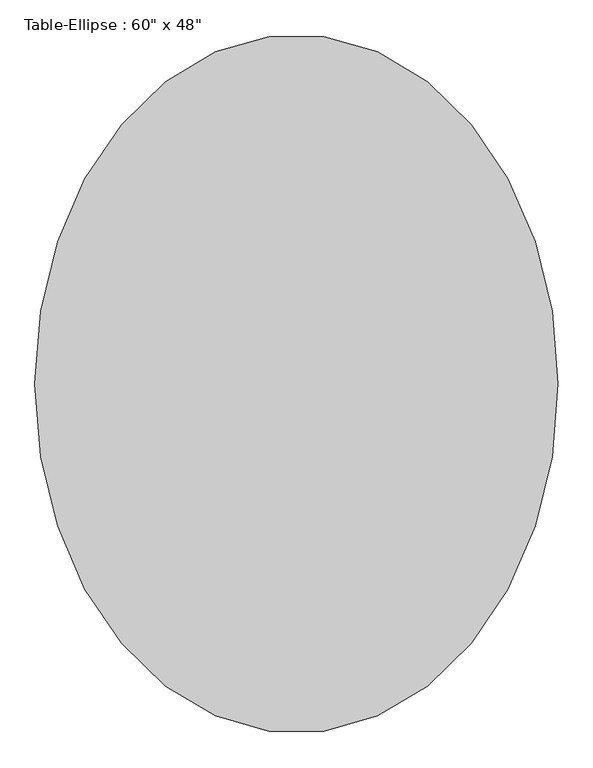
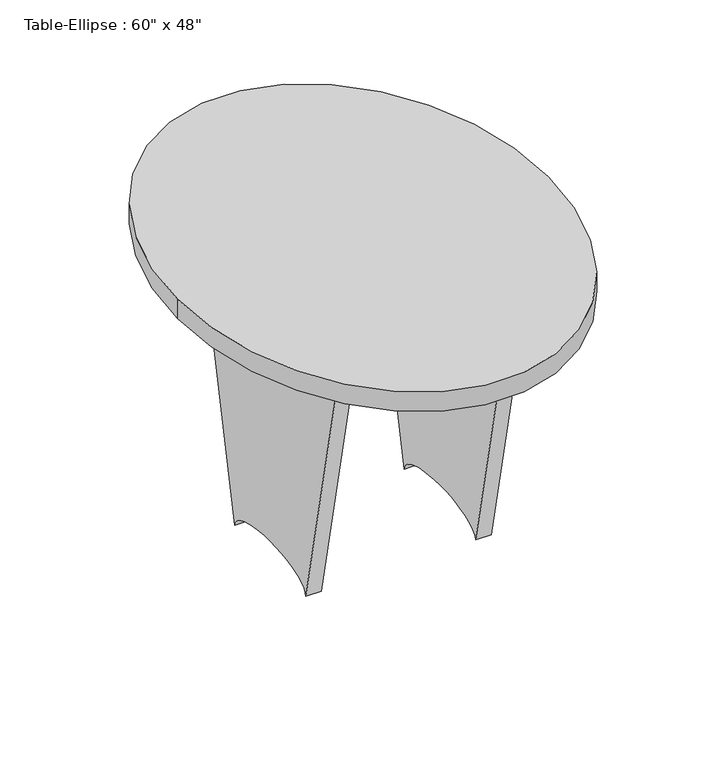
"""IFC4 building model written with IfcOpenShell, lengths in millimetres: furniture geometry."""

from ifc_helpers import new_model, si_unit, point, frame, origin, place, context, project, spatial, ellipse_curve, trimmed, source, transform, mapped, element, save
from ifc_brep_helpers import plane_surface, extruded_surface, advanced_brep


def furniture_b1c544a7(model_context):
    return source(origin(), model_context, "Body", "AdvancedBrep", [
        advanced_brep(
        [(-190.5, 19.05, 711.2), (190.5, 19.05, 711.2), (190.5, 19.05, 474.1333333), (-190.5, 19.05, 474.1333333), (-190.5, -19.05, 711.2), (-190.5, -19.05, 474.1333333), (190.5, -19.05, 474.1333333), (190.5, -19.05, 711.2)],
        [
            (0, 1),
            (1, 2),
            (2, 3, ellipse_curve(frame((0.0, 19.05, 474.1333333), z_axis=(0.0, -1.0, 0.0), x_axis=(1.0, 0.0, 0.0)), 190.5, 101.6)),
            (3, 0),
            (4, 5),
            (5, 6, ellipse_curve(frame((0.0, -19.05, 474.1333333), z_axis=(0.0, 1.0, 0.0), x_axis=(1.0, 0.0, 0.0)), 190.5, 101.6)),
            (6, 7),
            (7, 4),
            (0, 4),
            (7, 1),
            (6, 2),
            (5, 3),
        ],
        [
            plane_surface(frame((-190.5, 19.05, 711.2), z_axis=(0.0, 1.0, 0.0), x_axis=(1.0, 0.0, 0.0))),
            plane_surface(frame((-190.5, -19.05, 711.2), z_axis=(0.0, -1.0, 0.0), x_axis=(-1.0, 0.0, 0.0))),
            plane_surface(frame((-190.5, 19.05, 711.2), z_axis=(0.0, 0.0, 1.0), x_axis=(0.0, -1.0, 0.0))),
            plane_surface(frame((190.5, 19.05, 711.2), z_axis=(1.0, 0.0, 0.0), x_axis=(0.0, -1.0, 0.0))),
            extruded_surface(trimmed(ellipse_curve(frame((0.0, -57.15, 474.1333333), z_axis=(0.0, -1.0, 0.0), x_axis=(1.0, 0.0, 0.0)), 190.5, 101.6), [point((190.5, -57.15, 474.1333333))], [point((-190.5, -57.15, 474.1333333))], True, "CARTESIAN"), (0.0, 38.099999999999994, 0.0), 38.099999999999994),
            plane_surface(frame((-190.5, 19.05, 474.1333333), z_axis=(-1.0, 0.0, 0.0), x_axis=(0.0, -1.0, 0.0))),
        ],
        [
            (0, [[1, 2, 3, 4]]),
            (1, [[5, 6, 7, 8]]),
            (2, [[-1, 9, -8, 10]]),
            (3, [[-2, -10, -7, 11]]),
            (4, [[-3, -11, -6, 12]]),
            (5, [[-4, -12, -5, -9]]),
        ],
    ),
        advanced_brep(
        [(228.6, 304.8, 711.2), (228.6, -304.8, 711.2), (228.6, -152.4, 0.0), (228.6, 152.4, 0.0), (190.5, 304.8, 711.2), (190.5, 152.4, 0.0), (190.5, -152.4, 0.0), (190.5, -304.8, 711.2)],
        [
            (0, 1),
            (1, 2),
            (2, 3, ellipse_curve(frame((228.6, 0.0, 0.0), z_axis=(-1.0, 0.0, 0.0), x_axis=(0.0, 1.0, 0.0)), 152.4, 50.8)),
            (3, 0),
            (4, 5),
            (5, 6, ellipse_curve(frame((190.5, 0.0, 0.0), z_axis=(1.0, 0.0, 0.0), x_axis=(0.0, 1.0, 0.0)), 152.4, 50.8)),
            (6, 7),
            (7, 4),
            (0, 4),
            (7, 1),
            (6, 2),
            (5, 3),
        ],
        [
            plane_surface(frame((228.6, -304.8, 711.2), z_axis=(1.0, 0.0, 0.0), x_axis=(0.0, -1.0, 0.0))),
            plane_surface(frame((190.5, -304.8, 711.2), z_axis=(-1.0, 0.0, 0.0), x_axis=(0.0, 1.0, 0.0))),
            plane_surface(frame((228.6, 304.8, 711.2), z_axis=(0.0, 0.0, 1.0), x_axis=(-1.0, 0.0, 0.0))),
            plane_surface(frame((228.6, -304.8, 711.2), z_axis=(0.0, -0.9778024140774091, -0.2095290887308754), x_axis=(-1.0, 0.0, 0.0))),
            extruded_surface(trimmed(ellipse_curve(frame((152.4, 0.0, 0.0), z_axis=(-1.0, 0.0, 0.0), x_axis=(0.0, 1.0, 0.0)), 152.4, 50.8), [point((152.4, -152.4, 0.0))], [point((152.4, 152.4, 0.0))], True, "CARTESIAN"), (38.099999999999994, 0.0, 0.0), 38.099999999999994),
            plane_surface(frame((228.6, 152.4, 0.0), z_axis=(0.0, 0.977802414077412, -0.2095290887308621), x_axis=(-1.0, 0.0, 0.0))),
        ],
        [
            (0, [[1, 2, 3, 4]]),
            (1, [[5, 6, 7, 8]]),
            (2, [[-1, 9, -8, 10]]),
            (3, [[-2, -10, -7, 11]]),
            (4, [[-3, -11, -6, 12]]),
            (5, [[-4, -12, -5, -9]]),
        ],
    ),
        advanced_brep(
        [(-190.5, 304.8, 711.2), (-190.5, -304.8, 711.2), (-190.5, -152.4, 0.0), (-190.5, 152.4, 0.0), (-228.6, 304.8, 711.2), (-228.6, 152.4, 0.0), (-228.6, -152.4, 0.0), (-228.6, -304.8, 711.2)],
        [
            (0, 1),
            (1, 2),
            (2, 3, ellipse_curve(frame((-190.5, 0.0, 0.0), z_axis=(-1.0, 0.0, 0.0), x_axis=(0.0, 1.0, 0.0)), 152.4, 50.8)),
            (3, 0),
            (4, 5),
            (5, 6, ellipse_curve(frame((-228.6, 0.0, 0.0), z_axis=(1.0, 0.0, 0.0), x_axis=(0.0, 1.0, 0.0)), 152.4, 50.8)),
            (6, 7),
            (7, 4),
            (0, 4),
            (7, 1),
            (6, 2),
            (5, 3),
        ],
        [
            plane_surface(frame((-190.5, -304.8, 711.2), z_axis=(1.0, 0.0, 0.0), x_axis=(0.0, -1.0, 0.0))),
            plane_surface(frame((-228.6, -304.8, 711.2), z_axis=(-1.0, 0.0, 0.0), x_axis=(0.0, 1.0, 0.0))),
            plane_surface(frame((-190.5, 304.8, 711.2), z_axis=(0.0, 0.0, 1.0), x_axis=(-1.0, 0.0, 0.0))),
            plane_surface(frame((-190.5, -304.8, 711.2), z_axis=(0.0, -0.9778024140774088, -0.2095290887308767), x_axis=(-1.0, 0.0, 0.0))),
            extruded_surface(trimmed(ellipse_curve(frame((-266.7, 0.0, 0.0), z_axis=(-1.0, 0.0, 0.0), x_axis=(0.0, 1.0, 0.0)), 152.4, 50.8), [point((-266.7, -152.4, 0.0))], [point((-266.7, 152.4, 0.0))], True, "CARTESIAN"), (38.099999999999994, 0.0, 0.0), 38.099999999999994),
            plane_surface(frame((-190.5, 152.4, 0.0), z_axis=(0.0, 0.9778024140774109, -0.2095290887308677), x_axis=(-1.0, 0.0, 0.0))),
        ],
        [
            (0, [[1, 2, 3, 4]]),
            (1, [[5, 6, 7, 8]]),
            (2, [[-1, 9, -8, 10]]),
            (3, [[-2, -10, -7, 11]]),
            (4, [[-3, -11, -6, 12]]),
            (5, [[-4, -12, -5, -9]]),
        ],
    ),
        advanced_brep(
        [(-457.2, 0.0, 762.0), (457.2, 0.0, 762.0), (-457.2, 0.0, 711.2), (457.2, 0.0, 711.2)],
        [
            (0, 1, ellipse_curve(frame((0.0, 0.0, 762.0), z_axis=(0.0, 0.0, 1.0), x_axis=(0.0, 1.0, 0.0)), 609.6, 457.2)),
            (1, 0, ellipse_curve(frame((0.0, 0.0, 762.0), z_axis=(0.0, 0.0, 1.0), x_axis=(0.0, 1.0, 0.0)), 609.6, 457.2)),
            (2, 3, ellipse_curve(frame((0.0, 0.0, 711.2), z_axis=(0.0, 0.0, -1.0), x_axis=(1.0, 0.0, 0.0)), 457.2, 609.6)),
            (3, 2, ellipse_curve(frame((0.0, 0.0, 711.2), z_axis=(0.0, 0.0, -1.0), x_axis=(1.0, 0.0, 0.0)), 457.2, 609.6)),
            (0, 2),
            (3, 1),
        ],
        [
            plane_surface(frame((457.2, 0.0, 762.0), z_axis=(0.0, 0.0, 1.0), x_axis=(0.0, 1.0, 0.0))),
            plane_surface(frame((457.2, 0.0, 711.2), z_axis=(0.0, 0.0, -1.0), x_axis=(0.0, -1.0, 0.0))),
            extruded_surface(trimmed(ellipse_curve(frame((0.0, 0.0, 660.4), z_axis=(0.0, 0.0, 1.0), x_axis=(1.0, 0.0, 0.0)), 457.2, 609.6), [point((-457.2, 0.0, 660.4))], [point((457.2, 0.0, 660.4))], True, "CARTESIAN"), (0.0, 0.0, 50.80000000000007), 50.80000000000007),
            extruded_surface(trimmed(ellipse_curve(frame((0.0, 0.0, 660.4), z_axis=(0.0, 0.0, 1.0), x_axis=(1.0, 0.0, 0.0)), 457.2, 609.6), [point((457.2, 0.0, 660.4))], [point((-457.2, 0.0, 660.4))], True, "CARTESIAN"), (0.0, 0.0, 50.80000000000007), 50.80000000000007),
        ],
        [
            (0, [[1, 2]]),
            (1, [[3, 4]]),
            (2, [[-1, 5, -4, 6]]),
            (3, [[-2, -6, -3, -5]]),
        ],
    ),
    ])


if __name__ == "__main__":
    model = new_model("IFC4")
    model_context = context("Model", 3, world=origin())
    ifc_project = project(units=[si_unit("LENGTHUNIT", "METRE", prefix="MILLI")], contexts=[model_context])
    site = spatial("IfcSite", under=ifc_project)
    building = spatial("IfcBuilding", under=site)
    placement = place(None, origin())
    furniture_shape = furniture_b1c544a7(model_context)
    element("IfcFurniture", 1, ObjectType="Table-Ellipse : 60\" x 48\"", at=placement, inside=building, context=model_context, shape_type="MappedRepresentation", body=[
        mapped(furniture_shape, transform((0.0, 0.0, 0.0), x_axis=(1.0, 0.0, 0.0), y_axis=(0.0, 1.0, 0.0), z_axis=(0.0, 0.0, 1.0))),
    ])
    save(model, "model.ifc")

# Revit data of these elements
# Type "Table-Ellipse : 60\" x 48\""
#   Assembly Code = "E2020200"
#   Half Width = 2' - 0"
#   Half Length = 1' - 6"
#   Height = 2' - 6"
#   Length = 3' - 0"
#   Width = 4' - 0"
#   Base Material = Birch
#   Top Material = Birch
#   Default Elevation = 0
# Element 1 (IfcFurniture, "Table-Ellipse : 60\" x 48\"")
#   Materials on its faces: "Birch"
# Materials
#   "Birch": class "Wood", colour RGB 224 178 126, transparency 0, Description = "Betula Alleghaniensis", Cost = 0
